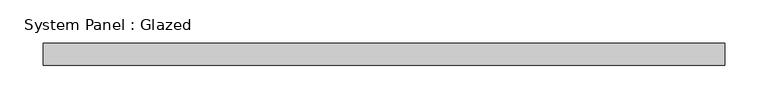
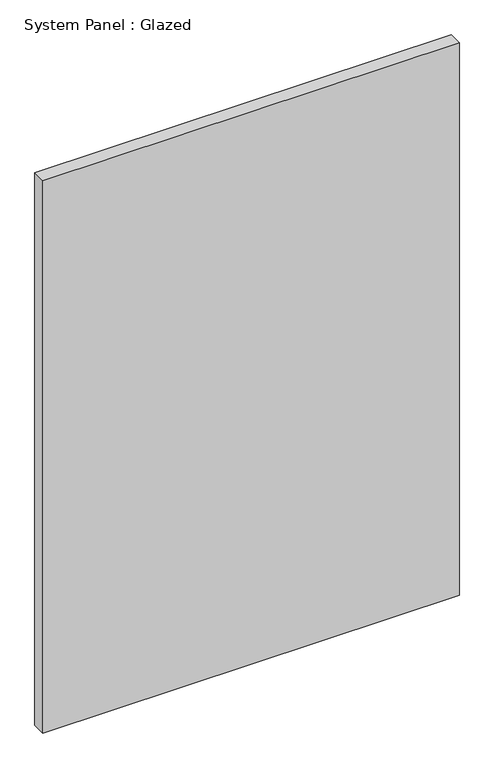
"""IFC4 building model written with IfcOpenShell, lengths in millimetres: plate geometry, System Panel : Glazed."""

from ifc_helpers import new_model, si_unit, origin, origin_with_axes, place, context, project, spatial, polyline, outline, extrude, source, transform, mapped, element, save


def system_panel_glazed_6fa9ab24(model_context):
    return source(origin(), model_context, "Body", "SweptSolid", [
        extrude(outline(polyline([(394.3296124, 19.05), (-394.3296124, 19.05), (-394.3296124, 44.45), (394.3296124, 44.45), (394.3296124, 19.05)])), origin_with_axes(), (0.0, 0.0, 1.0), 1104.9),
    ])


if __name__ == "__main__":
    model = new_model("IFC4")
    model_context = context("Model", 3, world=origin())
    ifc_project = project(units=[si_unit("LENGTHUNIT", "METRE", prefix="MILLI")], contexts=[model_context])
    site = spatial("IfcSite", under=ifc_project)
    building = spatial("IfcBuilding", under=site)
    placement = place(None, origin())
    system_panel_glazed_shape = system_panel_glazed_6fa9ab24(model_context)
    element("IfcPlate", 1, ObjectType="System Panel : Glazed", at=placement, inside=building, context=model_context, shape_type="MappedRepresentation", body=[
        mapped(system_panel_glazed_shape, transform((0.0, 0.0, 0.0), x_axis=(1.0, 0.0, 0.0), y_axis=(0.0, 1.0, 0.0), z_axis=(0.0, 0.0, 1.0))),
    ])
    save(model, "model.ifc")

# Revit data of these elements
# Type "System Panel : Glazed"
#   Construction Type Id = "GSP4R"
#   Analytic Construction = "1/8 in Pilkington single glazing"
#   Visual Light Transmittance = 0.9
#   Solar Heat Gain Coefficient = 0.86
#   Heat Transfer Coefficient (U) = 1.18115 BTU/(h·ft²·°F)
# Element 1 (IfcPlate, "System Panel : Glazed")
#   Materials on its faces: "Glass"
# Materials
#   "Glass": class "Glass", colour RGB 0 128 192, transparency 0.75, Description = "Soda Lime Glass", Cost = 0
